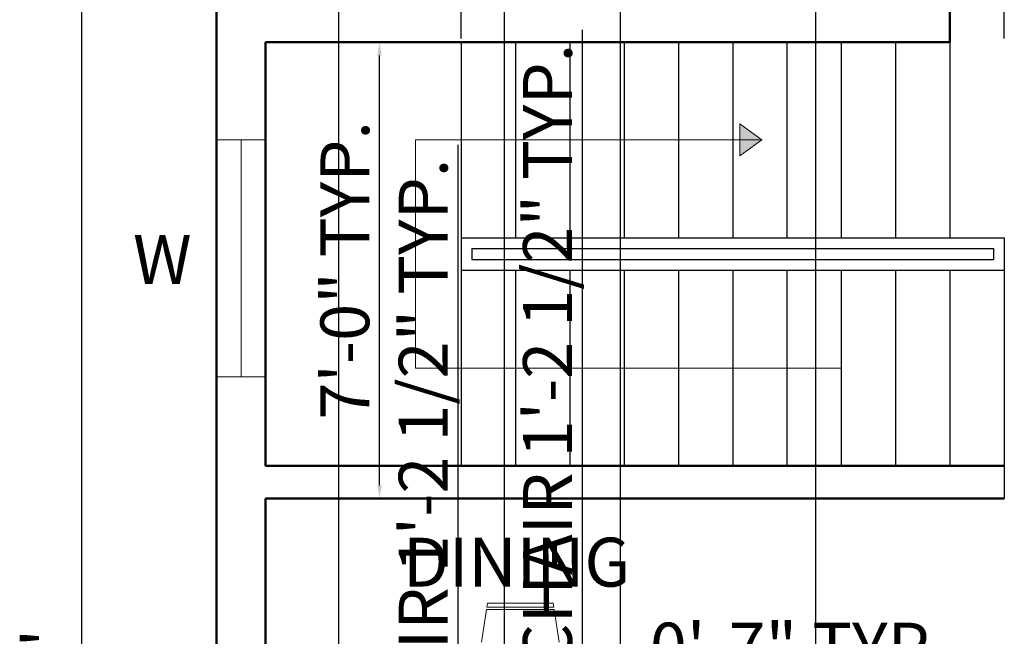
# Model space of a CAD drawing. Units: inches. Extents: x 3587 to 4539, y 1613 to 2440.
# Tile 4 of 8: x 3608 to 3790, y 2027 to 2140. Entities that reach past the tile are written whole.
import ezdxf

# ---------------------------------------------------------------- set-up
doc = ezdxf.new("R2010")
doc.units = ezdxf.units.IN
for name, color, linetype, lineweight in [('A-ANNO-DIMS', 2, 'Continuous', 18), ('A-ANNO-SYMB', 7, 'Continuous', 18), ('A-ANNO-TEXT', 7, 'Continuous', 18), ('A-AREA-IDEN', 7, 'Continuous', 25), ('A-FLOR-STRS', 7, 'Continuous', 25), ('A-FURN', 8, 'Continuous', 18), ('A-GLAZ', 4, 'Continuous', 20), ('A-WALL', 7, 'Continuous', 50)]:
    doc.layers.add(name, color=color, linetype=linetype, lineweight=lineweight)
doc.styles.get("Standard").update_dxf_attribs({"font": 'arial.ttf'})
doc.dimstyles.new('ISO-25', dxfattribs={"dimtxt": 9, "dimasz": 2.5, "dimexe": 1.25, "dimexo": 0.625, "dimtad": 1, "dimlunit": 3, "dimtxsty": 'Standard', "dimcen": 2.5, "dimadec": 0, "dimazin": 0, "dimtfac": 1, "dimtmove": 0, "dimatfit": 3, "dimfxl": 1, "dimarcsym": 0})

# ---------------------------------------------------------------- blocks, each defined once
blk = doc.blocks.new('*D14')
at = {"layer": 'A-ANNO-DIMS', "color": 0, "lineweight": -2, "transparency": 16777216}
for p, q in [((3643.9, 2372.93), (3618.39, 2372.93)), ((3619.64, 2370.43), (3619.64, 1655.43)), ((3643.9, 1652.93), (3618.39, 1652.93))]:
    blk.add_line(p, q, dxfattribs=at)
at = {"layer": 'A-ANNO-DIMS', "color": 0, "transparency": 16777216}
for points in [[(3619.22, 2370.43), (3620.05, 2370.43), (3619.64, 2372.93)], [(3619.22, 1655.43), (3620.05, 1655.43), (3619.64, 1652.93)]]:
    blk.add_solid(points, dxfattribs=at)
at = {"layer": 'Defpoints', "color": 0, "transparency": 16777216}
for p in [(3644.52, 2372.93), (3619.64, 1652.93), (3644.52, 1652.93)]:
    blk.add_point(p, dxfattribs=at)
at = {"layer": 'A-ANNO-DIMS', "color": 0, "transparency": 16777216, "insert": (3614.42, 2019.45), "char_height": 9, "attachment_point": 5, "rotation": 90}
blk.add_mtext("60'", dxfattribs=at)
blk = doc.blocks.new('STAIR-DOGLEG')
for p, q in [((0, 84), (0, 6)), ((10, 84), (10, 48)), ((20, 84), (20, 48)), ((30, 84), (30, 48)), ((40, 84), (40, 48)), ((50, 84), (50, 48)), ((60, 84), (60, 48)), ((70, 84), (70, 48)), ((80, 84), (80, 48)), ((90, 84), (90, 48)), ((0, 48), (100, 48)), ((100, 48), (100, 0)), ((2, 46), (98, 46)), ((2, 46), (2, 44)), ((98, 46), (98, 44)), ((2, 44), (98, 44)), ((0, 42), (100, 42)), ((10, 42), (10, 6)), ((20, 42), (20, 6)), ((30, 42), (30, 6)), ((40, 42), (40, 6)), ((50, 42), (50, 6)), ((60, 42), (60, 6)), ((70, 42), (70, 6)), ((80, 42), (80, 6)), ((90, 42), (90, 6))]:
    blk.add_line(p, q)
blk = doc.blocks.new('STAIR-PATH-ARROW')
h = blk.add_hatch(color=256)
h.dxf.hatch_style = 1
h.paths.add_polyline_path([(63.77, 42), (59.72, 42), (59.72, 39.06)])
h.paths.add_polyline_path([(59.72, 44.94), (59.72, 42), (63.77, 42)])
for p, q in [((63.77, 42), (59.72, 44.94)), ((59.72, 44.94), (59.72, 42)), ((0, 0), (0, 42)), ((0, 42), (63.77, 42)), ((63.77, 42), (59.72, 39.06)), ((59.72, 39.06), (59.72, 42)), ((78.41, 0), (0, 0))]:
    blk.add_line(p, q)
blk = doc.blocks.new('WINDOW-43_61IN')
for p, q in [((9, 43.61), (0, 43.61)), ((4.5, 0), (4.5, 43.61)), ((9, 0), (0, 0))]:
    blk.add_line(p, q)
blk = doc.blocks.new('DINING-CHAIR-END')
for p, q in [((0, 0), (0.94, 6.04)), ((13.37, 6.04), (0.94, 6.04)), ((1, 6.42), (1.12, 7.17)), ((1, 6.42), (13.32, 6.42)), ((13.2, 7.17), (1.12, 7.17)), ((13.2, 7.17), (13.32, 6.42)), ((13.38, 6.04), (14.32, 0))]:
    blk.add_line(p, q)
blk = doc.blocks.new('*D66')
at = {"layer": 'A-ANNO-DIMS', "color": 0, "lineweight": -2, "transparency": 16777216}
for p, q in [((3689.52, 2136.56), (3689.52, 2152.18)), ((3789.52, 2136.56), (3789.52, 2152.18)), ((3692.02, 2150.93), (3787.02, 2150.93))]:
    blk.add_line(p, q, dxfattribs=at)
at = {"layer": 'A-ANNO-DIMS', "color": 0, "transparency": 16777216}
for points in [[(3692.02, 2151.35), (3692.02, 2150.52), (3689.52, 2150.93)], [(3787.02, 2151.35), (3787.02, 2150.52), (3789.52, 2150.93)]]:
    blk.add_solid(points, dxfattribs=at)
at = {"layer": 'Defpoints', "color": 0, "transparency": 16777216}
for p in [(3789.52, 2150.93), (3689.52, 2135.93), (3789.52, 2135.93)]:
    blk.add_point(p, dxfattribs=at)
at = {"layer": 'A-ANNO-DIMS', "color": 0, "transparency": 16777216, "insert": (3739.52, 2156.21), "char_height": 9, "attachment_point": 5}
blk.add_mtext('STAIR 8\'-4" TYP.', dxfattribs=at)
blk = doc.blocks.new('*D67')
at = {"layer": 'A-ANNO-DIMS', "color": 0, "lineweight": -2, "transparency": 16777216}
for p, q in [((3688.9, 2135.93), (3673.27, 2135.93)), ((3674.52, 2054.43), (3674.52, 2133.43)), ((3688.9, 2051.93), (3673.27, 2051.93))]:
    blk.add_line(p, q, dxfattribs=at)
at = {"layer": 'A-ANNO-DIMS', "color": 0, "transparency": 16777216}
for points in [[(3674.11, 2133.43), (3674.94, 2133.43), (3674.52, 2135.93)], [(3674.11, 2054.43), (3674.94, 2054.43), (3674.52, 2051.93)]]:
    blk.add_solid(points, dxfattribs=at)
at = {"layer": 'Defpoints', "color": 0, "transparency": 16777216}
for p in [(3674.52, 2135.93), (3689.52, 2135.93), (3689.52, 2051.93)]:
    blk.add_point(p, dxfattribs=at)
at = {"layer": 'A-ANNO-DIMS', "color": 0, "transparency": 16777216, "insert": (3669.3, 2093.93), "char_height": 9, "attachment_point": 5, "rotation": 90}
blk.add_mtext('7\'-0" TYP.', dxfattribs=at)
blk = doc.blocks.new('*D74')
at = {"layer": 'A-ANNO-DIMS', "color": 0, "lineweight": -2, "transparency": 16777216}
for p, q in [((3711.88, 2016.07), (3711.88, 2138.15)), ((3713.4, 2016.07), (3710.63, 2016.07)), ((3711.88, 2004.25), (3711.88, 2013.57)), ((3713.4, 2001.75), (3710.63, 2001.75))]:
    blk.add_line(p, q, dxfattribs=at)
at = {"layer": 'A-ANNO-DIMS', "color": 0, "transparency": 16777216}
for points in [[(3711.46, 2013.57), (3712.29, 2013.57), (3711.88, 2016.07)], [(3711.46, 2004.25), (3712.29, 2004.25), (3711.88, 2001.75)]]:
    blk.add_solid(points, dxfattribs=at)
at = {"layer": 'Defpoints', "color": 0, "transparency": 16777216}
for p in [(3711.88, 2016.07), (3714.02, 2016.07), (3714.02, 2001.75)]:
    blk.add_point(p, dxfattribs=at)
at = {"layer": 'A-ANNO-DIMS', "color": 0, "transparency": 16777216, "insert": (3706.6, 2078.36), "char_height": 9, "attachment_point": 5, "rotation": 90}
blk.add_mtext('CHAIR 1\'-2 1/2" TYP.', dxfattribs=at)
blk = doc.blocks.new('*D75')
at = {"layer": 'A-ANNO-DIMS', "color": 0, "lineweight": -2, "transparency": 16777216}
for p, q in [((3714.02, 2016.69), (3714.02, 2019.46)), ((3721.2, 2016.69), (3721.2, 2019.46)), ((3716.52, 2018.21), (3718.7, 2018.21)), ((3721.2, 2018.21), (3779.81, 2018.21))]:
    blk.add_line(p, q, dxfattribs=at)
at = {"layer": 'A-ANNO-DIMS', "color": 0, "transparency": 16777216}
for points in [[(3716.52, 2018.63), (3716.52, 2017.8), (3714.02, 2018.21)], [(3718.7, 2018.63), (3718.7, 2017.8), (3721.2, 2018.21)]]:
    blk.add_solid(points, dxfattribs=at)
at = {"layer": 'Defpoints', "color": 0, "transparency": 16777216}
for p in [(3721.2, 2018.21), (3714.02, 2016.07), (3721.2, 2016.07)]:
    blk.add_point(p, dxfattribs=at)
at = {"layer": 'A-ANNO-DIMS', "color": 0, "transparency": 16777216, "insert": (3751.75, 2023.43), "char_height": 9, "attachment_point": 5}
blk.add_mtext('0\'-7" TYP.', dxfattribs=at)
blk = doc.blocks.new('*D76')
at = {"layer": 'A-ANNO-DIMS', "color": 0, "lineweight": -2, "transparency": 16777216}
for p, q in [((3689, 1994.93), (3689, 2117.02)), ((3687.48, 1994.93), (3690.25, 1994.93)), ((3689, 1983.11), (3689, 1992.43)), ((3687.48, 1980.61), (3690.25, 1980.61))]:
    blk.add_line(p, q, dxfattribs=at)
at = {"layer": 'A-ANNO-DIMS', "color": 0, "transparency": 16777216}
for points in [[(3688.58, 1992.43), (3689.42, 1992.43), (3689, 1994.93)], [(3688.58, 1983.11), (3689.42, 1983.11), (3689, 1980.61)]]:
    blk.add_solid(points, dxfattribs=at)
at = {"layer": 'Defpoints', "color": 0, "transparency": 16777216}
for p in [(3686.85, 1994.93), (3689, 1994.93), (3686.85, 1980.61)]:
    blk.add_point(p, dxfattribs=at)
at = {"layer": 'A-ANNO-DIMS', "color": 0, "transparency": 16777216, "insert": (3683.72, 2057.22), "char_height": 9, "attachment_point": 5, "rotation": 90}
blk.add_mtext('CHAIR 1\'-2 1/2" TYP.', dxfattribs=at)
blk = doc.blocks.new('*D96')
at = {"layer": 'A-ANNO-DIMS', "color": 0, "lineweight": -2, "transparency": 16777216}
for p, q in [((3667.04, 1858.35), (3667.04, 2413.28)), ((3697.55, 1858.35), (3697.55, 2413.28)), ((3669.54, 2412.03), (3695.05, 2412.03)), ((3697.55, 2412.03), (3746.35, 2412.03))]:
    blk.add_line(p, q, dxfattribs=at)
at = {"layer": 'A-ANNO-DIMS', "color": 0, "transparency": 16777216}
for points in [[(3669.54, 2412.45), (3669.54, 2411.62), (3667.04, 2412.03)], [(3695.05, 2412.45), (3695.05, 2411.62), (3697.55, 2412.03)]]:
    blk.add_solid(points, dxfattribs=at)
at = {"layer": 'Defpoints', "color": 0, "transparency": 16777216}
for p in [(3697.55, 2412.03), (3667.04, 1857.73), (3697.55, 1857.73)]:
    blk.add_point(p, dxfattribs=at)
at = {"layer": 'A-ANNO-DIMS', "color": 0, "transparency": 16777216, "insert": (3723.2, 2417.31), "char_height": 9, "attachment_point": 5}
blk.add_mtext('2\'-6 1/2"', dxfattribs=at)
blk = doc.blocks.new('*D98')
at = {"layer": 'A-ANNO-DIMS', "color": 0, "lineweight": -2, "transparency": 16777216}
for p, q in [((3718.85, 1857.52), (3718.85, 2413.28)), ((3754.85, 1857.52), (3754.85, 2413.28)), ((3721.35, 2412.03), (3752.35, 2412.03))]:
    blk.add_line(p, q, dxfattribs=at)
at = {"layer": 'A-ANNO-DIMS', "color": 0, "transparency": 16777216}
for points in [[(3721.35, 2412.45), (3721.35, 2411.62), (3718.85, 2412.03)], [(3752.35, 2412.45), (3752.35, 2411.62), (3754.85, 2412.03)]]:
    blk.add_solid(points, dxfattribs=at)
at = {"layer": 'Defpoints', "color": 0, "transparency": 16777216}
for p in [(3754.85, 2412.03), (3718.85, 1856.9), (3754.85, 1856.9)]:
    blk.add_point(p, dxfattribs=at)
at = {"layer": 'A-ANNO-DIMS', "color": 0, "transparency": 16777216, "insert": (3736.85, 2417.26), "char_height": 9, "attachment_point": 5}
blk.add_mtext('3\'-0"', dxfattribs=at)

msp = doc.modelspace()

# ---------------------------------------------------------------- linework, layer by layer
at = {"layer": 'A-WALL'}
for p, q in [((3644.523, 2372.933), (3644.523, 1652.933)), ((3779.523, 2213.933), (3779.523, 2135.933)), ((3779.523, 2135.933), (3653.523, 2135.933)), ((3653.523, 2135.933), (3653.523, 2057.933)), ((3789.523, 2057.933), (3653.523, 2057.933)), ((3789.523, 2051.933), (3653.523, 2051.933)), ((3653.523, 2051.933), (3653.523, 1835.933))]:
    msp.add_line(p, q, dxfattribs=at)

# ---------------------------------------------------------------- block references
at = {"layer": 'A-ANNO-SYMB'}
msp.add_blockref('STAIR-PATH-ARROW', (3681.111, 2075.933), dxfattribs=at)
at = {"layer": 'A-FLOR-STRS'}
msp.add_blockref('STAIR-DOGLEG', (3689.523, 2051.933), dxfattribs=at)
at = {"layer": 'A-FURN'}
msp.add_blockref('DINING-CHAIR-END', (3693.278, 2025.512), dxfattribs=at)
at = {"layer": 'A-GLAZ'}
msp.add_blockref('WINDOW-43_61IN', (3644.523, 2074.325), dxfattribs=at)

# ---------------------------------------------------------------- texts
at = {"layer": 'A-ANNO-TEXT', "insert": (3629.146, 2100.404), "char_height": 9, "attachment_point": 1}
msp.add_mtext_dynamic_manual_height_columns('W', width=47.85632, gutter_width=12.5, heights=[0], dxfattribs=at)
at = {"layer": 'A-AREA-IDEN', "insert": (3678.837, 2044.737), "char_height": 9, "attachment_point": 1}
msp.add_mtext_dynamic_manual_height_columns('DINING', width=107.21909, gutter_width=12.5, heights=[0], dxfattribs=at)

# ---------------------------------------------------------------- dimensions: what is measured, and where the dimension line sits
at = {"layer": 'A-ANNO-DIMS'}
for base, p1, p2, picture, middle in [((3697.551, 2412.033), (3667.042, 1857.729), (3697.551, 1857.729), '*D96', (3723.2, 2417.312)), ((3754.854, 2412.033), (3718.854, 1856.898), (3754.854, 1856.898), '*D98', (3736.854, 2417.256))]:
    dim = msp.add_linear_dim(base=base, p1=p1, p2=p2, dimstyle='ISO-25', override={"dimdec": 1, "dimlfac": 1, "dimrnd": 0, "dimzin": 1, "dimdsep": 46, "dimlunit": 4, "dimfrac": 2}, dxfattribs=at)
    dim.commit()
    dim.dimension.update_dxf_attribs({"geometry": picture, "text_midpoint": middle})
dim = msp.add_linear_dim(base=(3619.637, 1652.933), p1=(3644.523, 2372.933), p2=(3644.523, 1652.933), angle=90, dimstyle='ISO-25', override={"dimclrd": 0, "dimclre": 0, "dimclrt": 0}, dxfattribs=at)
dim.commit()
dim.dimension.update_dxf_attribs({"geometry": '*D14', "text_midpoint": (3619.637, 2019.453), "dimtype": 160})
for base, p1, p2, text, picture, middle in [((3789.523, 2150.933), (3689.523, 2135.933), (3789.523, 2135.933), 'STAIR <> TYP.', '*D66', (3739.523, 2156.212)), ((3721.198, 2018.214), (3714.025, 2016.066), (3721.198, 2016.066), '<> TYP.', '*D75', (3751.753, 2023.434))]:
    dim = msp.add_linear_dim(base=base, p1=p1, p2=p2, text=text, dimstyle='ISO-25', override={"dimdec": 1, "dimlfac": 1, "dimrnd": 0, "dimzin": 1, "dimdsep": 46, "dimlunit": 4, "dimfrac": 2}, dxfattribs=at)
    dim.commit()
    dim.dimension.update_dxf_attribs({"geometry": picture, "text_midpoint": middle})
for base, p1, p2, text, picture, middle in [((3711.877, 2016.066), (3714.025, 2001.746), (3714.025, 2016.066), 'CHAIR <> TYP.', '*D74', (3706.598, 2078.36)), ((3674.523, 2135.933), (3689.523, 2051.933), (3689.523, 2135.933), '<> TYP.', '*D67', (3669.303, 2093.933)), ((3689, 1994.929), (3686.852, 1980.609), (3686.852, 1994.929), 'CHAIR <> TYP.', '*D76', (3683.722, 2057.223))]:
    dim = msp.add_linear_dim(base=base, p1=p1, p2=p2, angle=90, text=text, dimstyle='ISO-25', override={"dimdec": 1, "dimlfac": 1, "dimrnd": 0, "dimzin": 1, "dimdsep": 46, "dimlunit": 4, "dimfrac": 2}, dxfattribs=at)
    dim.commit()
    dim.dimension.update_dxf_attribs({"geometry": picture, "text_midpoint": middle})

doc.saveas('drawing.dxf')
